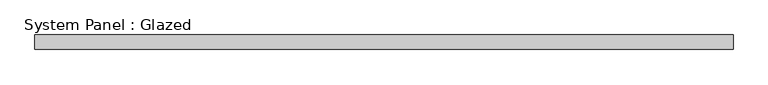
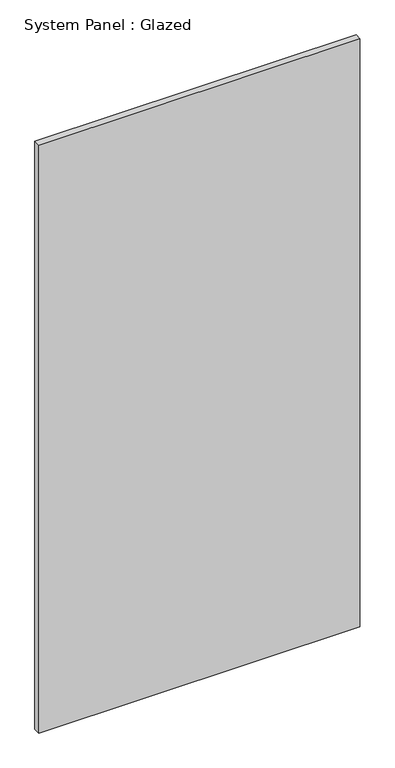
"""IFC4 building model written with IfcOpenShell, lengths in millimetres: plate geometry, System Panel : Glazed."""

from ifc_helpers import new_model, si_unit, origin, origin_with_axes, place, context, project, spatial, polyline, outline, extrude, source, transform, mapped, element, save


def system_panel_glazed_5eb7606f(model_context):
    return source(origin(), model_context, "Body", "SweptSolid", [
        extrude(outline(polyline([(613.4099999, 19.05), (-613.4099999, 19.05), (-613.4099999, 44.45), (613.4099999, 44.45), (613.4099999, 19.05)])), origin_with_axes(), (0.0, 0.0, 1.0), 2374.9),
    ])


if __name__ == "__main__":
    model = new_model("IFC4")
    model_context = context("Model", 3, world=origin())
    ifc_project = project(units=[si_unit("LENGTHUNIT", "METRE", prefix="MILLI")], contexts=[model_context])
    site = spatial("IfcSite", under=ifc_project)
    building = spatial("IfcBuilding", under=site)
    placement = place(None, origin())
    system_panel_glazed_shape = system_panel_glazed_5eb7606f(model_context)
    element("IfcPlate", 1, ObjectType="System Panel : Glazed", at=placement, inside=building, context=model_context, shape_type="MappedRepresentation", body=[
        mapped(system_panel_glazed_shape, transform((0.0, 0.0, 0.0), x_axis=(1.0, 0.0, 0.0), y_axis=(0.0, 1.0, 0.0), z_axis=(0.0, 0.0, 1.0))),
    ])
    save(model, "model.ifc")

# Revit data of these elements
# Type "System Panel : Glazed"
#   Construction Type Id = "GSP4R"
#   Analytic Construction = "1/8 in Pilkington single glazing"
#   Visual Light Transmittance = 0.9
#   Solar Heat Gain Coefficient = 0.86
#   Heat Transfer Coefficient (U) = 1.18115 BTU/(h·ft²·°F)
#   Define Thermal Properties by = 1
# Element 1 (IfcPlate, "System Panel : Glazed")
#   Materials on its faces: "Glass"
# Materials
#   "Glass": class "Glass", colour RGB 0 128 192, transparency 0.75, Description = "Soda Lime Glass", Cost = 0
